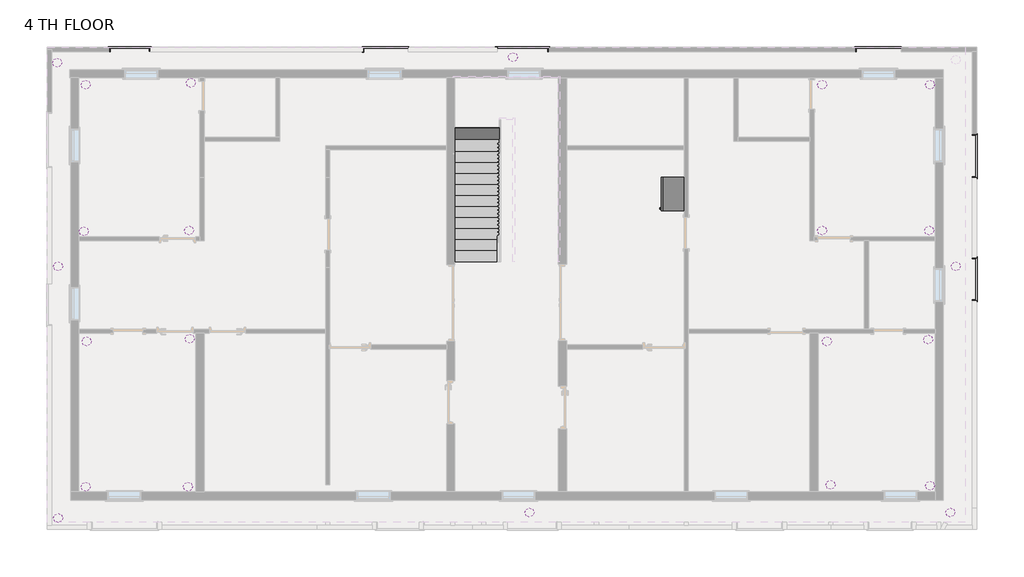
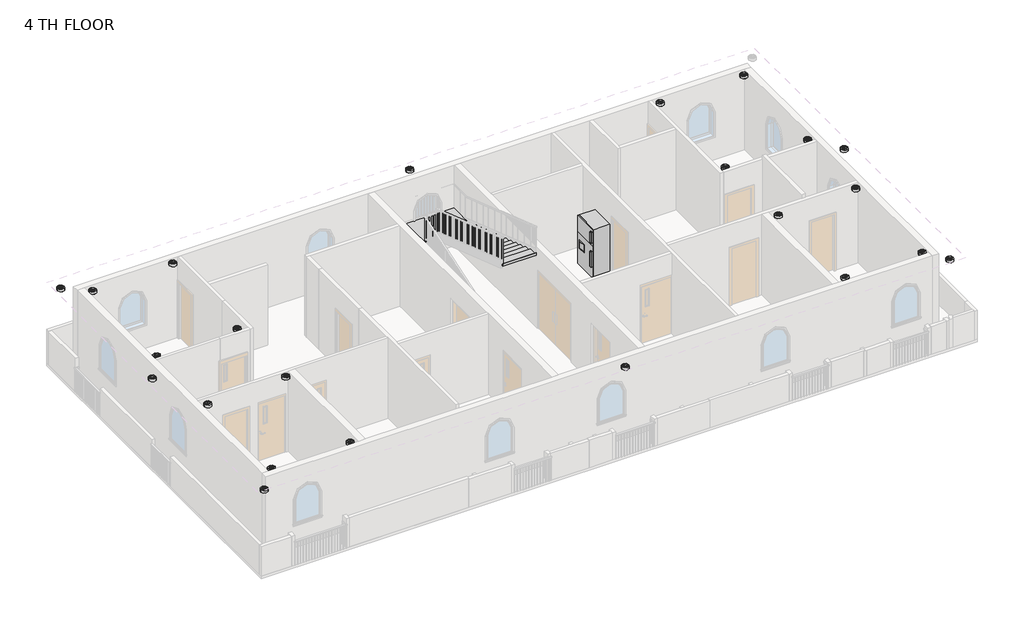
# One storey, part 6 of 7: 23 light fixtures, 6 railings, 1 furniture element, 1 stair flight.
# Revit data of these elements (continued)
# Element 21 (IfcLightFixture, "Ceiling Light - Flat Round : 60W - 120V") (continued)
#   Materials on its faces: "Glass, White, High Luminance", "Steel, Paint Finish, Dark Gray, Matte"
# Element 22 (IfcLightFixture, "Ceiling Light - Flat Round : 60W - 120V")
#   Mark = "133"
#   built-in parameter 1140040 = 1
#   Phase Created = New Construction
#   Materials on its faces: "Glass, White, High Luminance", "Steel, Paint Finish, Dark Gray, Matte"
# Element 23 (IfcLightFixture, "Ceiling Light - Flat Round : 60W - 120V")
#   Mark = "134"
#   built-in parameter 1140040 = 1
#   Phase Created = New Construction
#   Materials on its faces: "Glass, White, High Luminance", "Steel, Paint Finish, Dark Gray, Matte"
# Element 24 (IfcLightFixture, "Ceiling Light - Flat Round : 60W - 120V")
#   Mark = "135"
#   built-in parameter 1140040 = 1
#   Phase Created = New Construction
#   Materials on its faces: "Glass, White, High Luminance", "Steel, Paint Finish, Dark Gray, Matte"
# Elements 25, 26, 27, 28, 29, 30 (IfcRailing, "Handrail - Rectangular")
#   Phase Created = New Construction
# Element 31 (IfcStairFlight, "2\" Tread 1\" Nosing 1/4\" Riser")
#   Phase Created = New Construction
# Materials
#   "Steel, Paint Finish, Dark Gray, Matte": class "Metal", colour RGB 98 98 98, transparency 0, Description = "Steel, paint finish, dark gray, matte", Cost = 0
#   "Glass, White, High Luminance": class "Glass", colour RGB 249 250 249, transparency 0.8, Description = "physical material", Cost = 0
#   "Default": colour RGB 127 127 127, transparency 0, Cost = 0
#   "Default 3": class "Glass", colour RGB 127 127 127, transparency 0
#   "Default 2": class "Plastic", colour RGB 127 127 127, transparency 0
